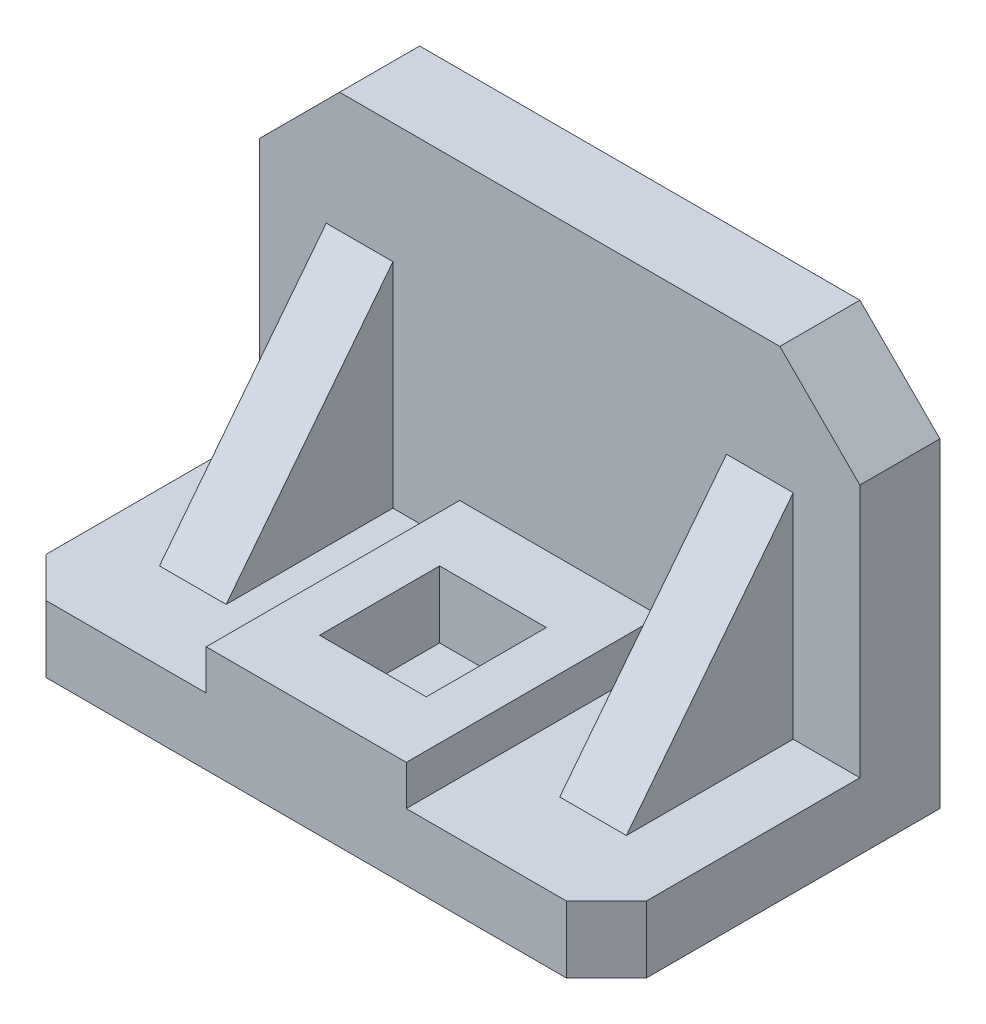
ISO-10303-21;
HEADER;
FILE_DESCRIPTION(('STEP AP214'),'2;1');
FILE_NAME('part.step','',(''),(''),'','','');
FILE_SCHEMA(('AUTOMOTIVE_DESIGN { 1 0 10303 214 1 1 1 1 }'));
ENDSEC;
DATA;
#1=APPLICATION_CONTEXT('core data for automotive mechanical design processes');
#2=APPLICATION_PROTOCOL_DEFINITION('international standard','automotive_design',2000,#1);
#3=PRODUCT_CONTEXT('',#1,'mechanical');
#4=PRODUCT('Part','Part','',(#3));
#5=PRODUCT_RELATED_PRODUCT_CATEGORY('part','',(#4));
#6=PRODUCT_DEFINITION_FORMATION('','',#4);
#7=PRODUCT_DEFINITION_CONTEXT('part definition',#1,'design');
#8=PRODUCT_DEFINITION('design','',#6,#7);
#9=PRODUCT_DEFINITION_SHAPE('','',#8);
#10=(LENGTH_UNIT() NAMED_UNIT(*) SI_UNIT(.MILLI.,.METRE.));
#11=(NAMED_UNIT(*) PLANE_ANGLE_UNIT() SI_UNIT($,.RADIAN.));
#12=(NAMED_UNIT(*) SI_UNIT($,.STERADIAN.) SOLID_ANGLE_UNIT());
#13=UNCERTAINTY_MEASURE_WITH_UNIT(LENGTH_MEASURE(1.E-05),#10,'distance_accuracy_value','');
#14=(GEOMETRIC_REPRESENTATION_CONTEXT(3) GLOBAL_UNCERTAINTY_ASSIGNED_CONTEXT((#13)) GLOBAL_UNIT_ASSIGNED_CONTEXT((#10,
#11,#12)) REPRESENTATION_CONTEXT('',''));
#15=CARTESIAN_POINT('',(0.,0.,0.));
#16=DIRECTION('',(0.,0.,1.));
#17=DIRECTION('',(1.,0.,0.));
#18=AXIS2_PLACEMENT_3D('',#15,#16,#17);
#19=CARTESIAN_POINT('',(70.,10.,37.));
#20=DIRECTION('',(0.,0.615644041972315,0.788024373724563));
#21=DIRECTION('',(0.,-0.788024373724563,0.615644041972315));
#22=AXIS2_PLACEMENT_3D('',#19,#20,#21);
#23=PLANE('',#22);
#24=DIRECTION('',(1.,0.,0.));
#25=VECTOR('',#24,1.);
#26=CARTESIAN_POINT('',(70.,10.,37.));
#27=LINE('',#26,#25);
#28=CARTESIAN_POINT('',(70.,10.,37.));
#29=VERTEX_POINT('',#28);
#30=CARTESIAN_POINT('',(80.,10.,37.));
#31=VERTEX_POINT('',#30);
#32=EDGE_CURVE('E422',#29,#31,#27,.T.);
#33=ORIENTED_EDGE('',*,*,#32,.T.);
#34=DIRECTION('',(0.,-0.788024373724563,0.615644041972315));
#35=VECTOR('',#34,1.);
#36=CARTESIAN_POINT('',(80.,10.,37.));
#37=LINE('',#36,#35);
#38=CARTESIAN_POINT('',(80.,42.,12.));
#39=VERTEX_POINT('',#38);
#40=EDGE_CURVE('E441',#39,#31,#37,.T.);
#41=ORIENTED_EDGE('',*,*,#40,.F.);
#42=DIRECTION('',(1.,0.,0.));
#43=VECTOR('',#42,1.);
#44=CARTESIAN_POINT('',(70.,42.,12.));
#45=LINE('',#44,#43);
#46=CARTESIAN_POINT('',(70.,42.,12.));
#47=VERTEX_POINT('',#46);
#48=EDGE_CURVE('E424',#47,#39,#45,.T.);
#49=ORIENTED_EDGE('',*,*,#48,.F.);
#50=DIRECTION('',(0.,-0.788024373724563,0.615644041972315));
#51=VECTOR('',#50,1.);
#52=CARTESIAN_POINT('',(70.,10.,37.));
#53=LINE('',#52,#51);
#54=EDGE_CURVE('E426',#47,#29,#53,.T.);
#55=ORIENTED_EDGE('',*,*,#54,.T.);
#56=EDGE_LOOP('',(#33,#41,#49,#55));
#57=FACE_BOUND('',#56,.T.);
#58=ADVANCED_FACE('F44',(#57),#23,.T.);
#59=CARTESIAN_POINT('',(0.,0.,12.));
#60=DIRECTION('',(0.,0.,-1.));
#61=DIRECTION('',(-1.,0.,0.));
#62=AXIS2_PLACEMENT_3D('',#59,#60,#61);
#63=PLANE('',#62);
#64=DIRECTION('',(0.,1.,0.));
#65=VECTOR('',#64,1.);
#66=CARTESIAN_POINT('',(70.,10.,12.));
#67=LINE('',#66,#65);
#68=CARTESIAN_POINT('',(70.,10.,12.));
#69=VERTEX_POINT('',#68);
#70=EDGE_CURVE('E433',#69,#47,#67,.T.);
#71=ORIENTED_EDGE('',*,*,#70,.T.);
#72=ORIENTED_EDGE('',*,*,#48,.T.);
#73=DIRECTION('',(0.,1.,0.));
#74=VECTOR('',#73,1.);
#75=CARTESIAN_POINT('',(80.,42.,12.));
#76=LINE('',#75,#74);
#77=CARTESIAN_POINT('',(80.,10.,12.));
#78=VERTEX_POINT('',#77);
#79=EDGE_CURVE('E70',#78,#39,#76,.T.);
#80=ORIENTED_EDGE('',*,*,#79,.F.);
#81=DIRECTION('',(1.,0.,0.));
#82=VECTOR('',#81,1.);
#83=CARTESIAN_POINT('',(80.,10.,12.));
#84=LINE('',#83,#82);
#85=CARTESIAN_POINT('',(90.,10.,12.));
#86=VERTEX_POINT('',#85);
#87=EDGE_CURVE('E381',#78,#86,#84,.T.);
#88=ORIENTED_EDGE('',*,*,#87,.T.);
#89=DIRECTION('',(0.,1.,0.));
#90=VECTOR('',#89,1.);
#91=CARTESIAN_POINT('',(90.,48.,12.));
#92=LINE('',#91,#90);
#93=CARTESIAN_POINT('',(90.,48.,12.));
#94=VERTEX_POINT('',#93);
#95=EDGE_CURVE('E326',#86,#94,#92,.T.);
#96=ORIENTED_EDGE('',*,*,#95,.T.);
#97=DIRECTION('',(-0.707106781186548,0.707106781186547,0.));
#98=VECTOR('',#97,1.);
#99=CARTESIAN_POINT('',(90.,48.,12.));
#100=LINE('',#99,#98);
#101=CARTESIAN_POINT('',(78.,60.,12.));
#102=VERTEX_POINT('',#101);
#103=EDGE_CURVE('E328',#94,#102,#100,.T.);
#104=ORIENTED_EDGE('',*,*,#103,.T.);
#105=DIRECTION('',(-1.,0.,0.));
#106=VECTOR('',#105,1.);
#107=CARTESIAN_POINT('',(12.,60.,12.));
#108=LINE('',#107,#106);
#109=CARTESIAN_POINT('',(12.,60.,12.));
#110=VERTEX_POINT('',#109);
#111=EDGE_CURVE('E335',#102,#110,#108,.T.);
#112=ORIENTED_EDGE('',*,*,#111,.T.);
#113=DIRECTION('',(-0.707106781186548,-0.707106781186548,0.));
#114=VECTOR('',#113,1.);
#115=CARTESIAN_POINT('',(0.,48.,12.));
#116=LINE('',#115,#114);
#117=CARTESIAN_POINT('',(0.,48.,12.));
#118=VERTEX_POINT('',#117);
#119=EDGE_CURVE('E332',#110,#118,#116,.T.);
#120=ORIENTED_EDGE('',*,*,#119,.T.);
#121=DIRECTION('',(0.,-1.,0.));
#122=VECTOR('',#121,1.);
#123=CARTESIAN_POINT('',(0.,0.,12.));
#124=LINE('',#123,#122);
#125=CARTESIAN_POINT('',(0.,10.,12.));
#126=VERTEX_POINT('',#125);
#127=EDGE_CURVE('E337',#118,#126,#124,.T.);
#128=ORIENTED_EDGE('',*,*,#127,.T.);
#129=DIRECTION('',(-1.,0.,0.));
#130=VECTOR('',#129,1.);
#131=CARTESIAN_POINT('',(10.,10.,12.));
#132=LINE('',#131,#130);
#133=CARTESIAN_POINT('',(10.,10.,12.));
#134=VERTEX_POINT('',#133);
#135=EDGE_CURVE('E213',#134,#126,#132,.T.);
#136=ORIENTED_EDGE('',*,*,#135,.F.);
#137=DIRECTION('',(0.,-1.,0.));
#138=VECTOR('',#137,1.);
#139=CARTESIAN_POINT('',(10.,42.,12.));
#140=LINE('',#139,#138);
#141=CARTESIAN_POINT('',(10.,42.,12.));
#142=VERTEX_POINT('',#141);
#143=EDGE_CURVE('E206',#142,#134,#140,.T.);
#144=ORIENTED_EDGE('',*,*,#143,.F.);
#145=DIRECTION('',(-1.,0.,0.));
#146=VECTOR('',#145,1.);
#147=CARTESIAN_POINT('',(20.,42.,12.));
#148=LINE('',#147,#146);
#149=CARTESIAN_POINT('',(20.,42.,12.));
#150=VERTEX_POINT('',#149);
#151=EDGE_CURVE('E212',#150,#142,#148,.T.);
#152=ORIENTED_EDGE('',*,*,#151,.F.);
#153=DIRECTION('',(0.,-1.,0.));
#154=VECTOR('',#153,1.);
#155=CARTESIAN_POINT('',(20.,10.,12.));
#156=LINE('',#155,#154);
#157=CARTESIAN_POINT('',(20.,10.,12.));
#158=VERTEX_POINT('',#157);
#159=EDGE_CURVE('E235',#150,#158,#156,.T.);
#160=ORIENTED_EDGE('',*,*,#159,.T.);
#161=DIRECTION('',(1.,0.,0.));
#162=VECTOR('',#161,1.);
#163=CARTESIAN_POINT('',(90.,10.,12.));
#164=LINE('',#163,#162);
#165=CARTESIAN_POINT('',(30.,10.,12.));
#166=VERTEX_POINT('',#165);
#167=EDGE_CURVE('E294',#158,#166,#164,.T.);
#168=ORIENTED_EDGE('',*,*,#167,.T.);
#169=DIRECTION('',(0.,-1.,0.));
#170=VECTOR('',#169,1.);
#171=CARTESIAN_POINT('',(30.,16.,12.));
#172=LINE('',#171,#170);
#173=CARTESIAN_POINT('',(30.,16.,12.));
#174=VERTEX_POINT('',#173);
#175=EDGE_CURVE('E280',#174,#166,#172,.T.);
#176=ORIENTED_EDGE('',*,*,#175,.F.);
#177=DIRECTION('',(-1.,0.,0.));
#178=VECTOR('',#177,1.);
#179=CARTESIAN_POINT('',(30.,16.,12.));
#180=LINE('',#179,#178);
#181=CARTESIAN_POINT('',(60.,16.,12.));
#182=VERTEX_POINT('',#181);
#183=EDGE_CURVE('E273',#182,#174,#180,.T.);
#184=ORIENTED_EDGE('',*,*,#183,.F.);
#185=DIRECTION('',(0.,-1.,0.));
#186=VECTOR('',#185,1.);
#187=CARTESIAN_POINT('',(60.,16.,12.));
#188=LINE('',#187,#186);
#189=CARTESIAN_POINT('',(60.,10.,12.));
#190=VERTEX_POINT('',#189);
#191=EDGE_CURVE('E285',#182,#190,#188,.T.);
#192=ORIENTED_EDGE('',*,*,#191,.T.);
#193=EDGE_CURVE('E291',#190,#69,#164,.T.);
#194=ORIENTED_EDGE('',*,*,#193,.T.);
#195=EDGE_LOOP('',(#71,#72,#80,#88,#96,#104,#112,#120,#128,#136,#144,#152,#160,#168,#176,#184,
#192,#194));
#196=FACE_BOUND('',#195,.T.);
#197=ADVANCED_FACE('F209',(#196),#63,.F.);
#198=CARTESIAN_POINT('',(0.,10.,0.));
#199=DIRECTION('',(0.,1.,0.));
#200=DIRECTION('',(0.,0.,1.));
#201=AXIS2_PLACEMENT_3D('',#198,#199,#200);
#202=PLANE('',#201);
#203=DIRECTION('',(-1.,0.,0.));
#204=VECTOR('',#203,1.);
#205=CARTESIAN_POINT('',(20.,10.,37.));
#206=LINE('',#205,#204);
#207=CARTESIAN_POINT('',(20.,10.,37.));
#208=VERTEX_POINT('',#207);
#209=CARTESIAN_POINT('',(10.,10.,37.));
#210=VERTEX_POINT('',#209);
#211=EDGE_CURVE('E226',#208,#210,#206,.T.);
#212=ORIENTED_EDGE('',*,*,#211,.T.);
#213=DIRECTION('',(0.,0.,1.));
#214=VECTOR('',#213,1.);
#215=CARTESIAN_POINT('',(10.,10.,12.));
#216=LINE('',#215,#214);
#217=EDGE_CURVE('E58',#134,#210,#216,.T.);
#218=ORIENTED_EDGE('',*,*,#217,.F.);
#219=ORIENTED_EDGE('',*,*,#135,.T.);
#220=DIRECTION('',(0.,0.,-1.));
#221=VECTOR('',#220,1.);
#222=CARTESIAN_POINT('',(0.,10.,12.));
#223=LINE('',#222,#221);
#224=CARTESIAN_POINT('',(0.,10.,44.));
#225=VERTEX_POINT('',#224);
#226=EDGE_CURVE('E293',#225,#126,#223,.T.);
#227=ORIENTED_EDGE('',*,*,#226,.F.);
#228=DIRECTION('',(-0.707106781186547,0.,-0.707106781186548));
#229=VECTOR('',#228,1.);
#230=CARTESIAN_POINT('',(0.,10.,44.));
#231=LINE('',#230,#229);
#232=CARTESIAN_POINT('',(6.,10.,50.));
#233=VERTEX_POINT('',#232);
#234=EDGE_CURVE('E306',#233,#225,#231,.T.);
#235=ORIENTED_EDGE('',*,*,#234,.F.);
#236=DIRECTION('',(-1.,0.,0.));
#237=VECTOR('',#236,1.);
#238=CARTESIAN_POINT('',(6.,10.,50.));
#239=LINE('',#238,#237);
#240=CARTESIAN_POINT('',(30.,10.,50.));
#241=VERTEX_POINT('',#240);
#242=EDGE_CURVE('E305',#241,#233,#239,.T.);
#243=ORIENTED_EDGE('',*,*,#242,.F.);
#244=DIRECTION('',(0.,0.,1.));
#245=VECTOR('',#244,1.);
#246=CARTESIAN_POINT('',(30.,10.,12.));
#247=LINE('',#246,#245);
#248=EDGE_CURVE('E258',#166,#241,#247,.T.);
#249=ORIENTED_EDGE('',*,*,#248,.F.);
#250=ORIENTED_EDGE('',*,*,#167,.F.);
#251=DIRECTION('',(0.,0.,1.));
#252=VECTOR('',#251,1.);
#253=CARTESIAN_POINT('',(20.,10.,12.));
#254=LINE('',#253,#252);
#255=EDGE_CURVE('E423',#158,#208,#254,.T.);
#256=ORIENTED_EDGE('',*,*,#255,.T.);
#257=EDGE_LOOP('',(#212,#218,#219,#227,#235,#243,#249,#250,#256));
#258=FACE_BOUND('',#257,.T.);
#259=ADVANCED_FACE('F401',(#258),#202,.T.);
#260=ORIENTED_EDGE('',*,*,#32,.F.);
#261=DIRECTION('',(0.,0.,-1.));
#262=VECTOR('',#261,1.);
#263=CARTESIAN_POINT('',(70.,10.,12.));
#264=LINE('',#263,#262);
#265=EDGE_CURVE('E434',#29,#69,#264,.T.);
#266=ORIENTED_EDGE('',*,*,#265,.T.);
#267=ORIENTED_EDGE('',*,*,#193,.F.);
#268=DIRECTION('',(0.,0.,-1.));
#269=VECTOR('',#268,1.);
#270=CARTESIAN_POINT('',(60.,10.,12.));
#271=LINE('',#270,#269);
#272=CARTESIAN_POINT('',(60.,10.,50.));
#273=VERTEX_POINT('',#272);
#274=EDGE_CURVE('E272',#273,#190,#271,.T.);
#275=ORIENTED_EDGE('',*,*,#274,.F.);
#276=CARTESIAN_POINT('',(84.,10.,50.));
#277=VERTEX_POINT('',#276);
#278=EDGE_CURVE('E303',#277,#273,#239,.T.);
#279=ORIENTED_EDGE('',*,*,#278,.F.);
#280=DIRECTION('',(-0.707106781186547,0.,0.707106781186547));
#281=VECTOR('',#280,1.);
#282=CARTESIAN_POINT('',(90.,10.,44.));
#283=LINE('',#282,#281);
#284=CARTESIAN_POINT('',(90.,10.,44.));
#285=VERTEX_POINT('',#284);
#286=EDGE_CURVE('E299',#285,#277,#283,.T.);
#287=ORIENTED_EDGE('',*,*,#286,.F.);
#288=DIRECTION('',(0.,0.,1.));
#289=VECTOR('',#288,1.);
#290=CARTESIAN_POINT('',(90.,10.,12.));
#291=LINE('',#290,#289);
#292=EDGE_CURVE('E300',#86,#285,#291,.T.);
#293=ORIENTED_EDGE('',*,*,#292,.F.);
#294=ORIENTED_EDGE('',*,*,#87,.F.);
#295=DIRECTION('',(0.,0.,-1.));
#296=VECTOR('',#295,1.);
#297=CARTESIAN_POINT('',(80.,10.,12.));
#298=LINE('',#297,#296);
#299=EDGE_CURVE('E437',#31,#78,#298,.T.);
#300=ORIENTED_EDGE('',*,*,#299,.F.);
#301=EDGE_LOOP('',(#260,#266,#267,#275,#279,#287,#293,#294,#300));
#302=FACE_BOUND('',#301,.T.);
#303=ADVANCED_FACE('F388',(#302),#202,.T.);
#304=CARTESIAN_POINT('',(90.,0.,12.));
#305=DIRECTION('',(0.,1.,0.));
#306=DIRECTION('',(0.,0.,1.));
#307=AXIS2_PLACEMENT_3D('',#304,#305,#306);
#308=PLANE('',#307);
#309=DIRECTION('',(1.,0.,0.));
#310=VECTOR('',#309,1.);
#311=CARTESIAN_POINT('',(90.,0.,0.));
#312=LINE('',#311,#310);
#313=CARTESIAN_POINT('',(0.,0.,0.));
#314=VERTEX_POINT('',#313);
#315=CARTESIAN_POINT('',(90.,0.,0.));
#316=VERTEX_POINT('',#315);
#317=EDGE_CURVE('E318',#314,#316,#312,.T.);
#318=ORIENTED_EDGE('',*,*,#317,.T.);
#319=DIRECTION('',(0.,0.,-1.));
#320=VECTOR('',#319,1.);
#321=CARTESIAN_POINT('',(90.,0.,12.));
#322=LINE('',#321,#320);
#323=CARTESIAN_POINT('',(90.,0.,44.));
#324=VERTEX_POINT('',#323);
#325=EDGE_CURVE('E11',#324,#316,#322,.T.);
#326=ORIENTED_EDGE('',*,*,#325,.F.);
#327=DIRECTION('',(-0.707106781186547,0.,0.707106781186547));
#328=VECTOR('',#327,1.);
#329=CARTESIAN_POINT('',(90.,0.,44.));
#330=LINE('',#329,#328);
#331=CARTESIAN_POINT('',(84.,0.,50.));
#332=VERTEX_POINT('',#331);
#333=EDGE_CURVE('E289',#324,#332,#330,.T.);
#334=ORIENTED_EDGE('',*,*,#333,.T.);
#335=DIRECTION('',(-1.,0.,0.));
#336=VECTOR('',#335,1.);
#337=CARTESIAN_POINT('',(6.,0.,50.));
#338=LINE('',#337,#336);
#339=CARTESIAN_POINT('',(6.,0.,50.));
#340=VERTEX_POINT('',#339);
#341=EDGE_CURVE('E315',#332,#340,#338,.T.);
#342=ORIENTED_EDGE('',*,*,#341,.T.);
#343=DIRECTION('',(-0.707106781186547,0.,-0.707106781186548));
#344=VECTOR('',#343,1.);
#345=CARTESIAN_POINT('',(0.,0.,44.));
#346=LINE('',#345,#344);
#347=CARTESIAN_POINT('',(0.,0.,44.));
#348=VERTEX_POINT('',#347);
#349=EDGE_CURVE('E295',#340,#348,#346,.T.);
#350=ORIENTED_EDGE('',*,*,#349,.T.);
#351=DIRECTION('',(0.,0.,-1.));
#352=VECTOR('',#351,1.);
#353=CARTESIAN_POINT('',(0.,0.,12.));
#354=LINE('',#353,#352);
#355=EDGE_CURVE('E336',#348,#314,#354,.T.);
#356=ORIENTED_EDGE('',*,*,#355,.T.);
#357=EDGE_LOOP('',(#318,#326,#334,#342,#350,#356));
#358=FACE_BOUND('',#357,.T.);
#359=ADVANCED_FACE('F50',(#358),#308,.F.);
#360=CARTESIAN_POINT('',(90.,48.,12.));
#361=DIRECTION('',(-1.,0.,0.));
#362=DIRECTION('',(0.,0.,1.));
#363=AXIS2_PLACEMENT_3D('',#360,#361,#362);
#364=PLANE('',#363);
#365=ORIENTED_EDGE('',*,*,#95,.F.);
#366=ORIENTED_EDGE('',*,*,#292,.T.);
#367=DIRECTION('',(0.,-1.,0.));
#368=VECTOR('',#367,1.);
#369=CARTESIAN_POINT('',(90.,10.,44.));
#370=LINE('',#369,#368);
#371=EDGE_CURVE('E307',#285,#324,#370,.T.);
#372=ORIENTED_EDGE('',*,*,#371,.T.);
#373=ORIENTED_EDGE('',*,*,#325,.T.);
#374=DIRECTION('',(0.,1.,0.));
#375=VECTOR('',#374,1.);
#376=CARTESIAN_POINT('',(90.,48.,0.));
#377=LINE('',#376,#375);
#378=CARTESIAN_POINT('',(90.,48.,0.));
#379=VERTEX_POINT('',#378);
#380=EDGE_CURVE('E342',#316,#379,#377,.T.);
#381=ORIENTED_EDGE('',*,*,#380,.T.);
#382=DIRECTION('',(0.,0.,-1.));
#383=VECTOR('',#382,1.);
#384=CARTESIAN_POINT('',(90.,48.,12.));
#385=LINE('',#384,#383);
#386=EDGE_CURVE('E52',#94,#379,#385,.T.);
#387=ORIENTED_EDGE('',*,*,#386,.F.);
#388=EDGE_LOOP('',(#365,#366,#372,#373,#381,#387));
#389=FACE_BOUND('',#388,.T.);
#390=ADVANCED_FACE('F387',(#389),#364,.F.);
#391=CARTESIAN_POINT('',(90.,48.,12.));
#392=DIRECTION('',(-0.707106781186547,-0.707106781186548,0.));
#393=DIRECTION('',(0.707106781186548,-0.707106781186547,0.));
#394=AXIS2_PLACEMENT_3D('',#391,#392,#393);
#395=PLANE('',#394);
#396=DIRECTION('',(-0.707106781186548,0.707106781186547,0.));
#397=VECTOR('',#396,1.);
#398=CARTESIAN_POINT('',(90.,48.,0.));
#399=LINE('',#398,#397);
#400=CARTESIAN_POINT('',(78.,60.,0.));
#401=VERTEX_POINT('',#400);
#402=EDGE_CURVE('E344',#379,#401,#399,.T.);
#403=ORIENTED_EDGE('',*,*,#402,.T.);
#404=DIRECTION('',(0.,0.,-1.));
#405=VECTOR('',#404,1.);
#406=CARTESIAN_POINT('',(78.,60.,12.));
#407=LINE('',#406,#405);
#408=EDGE_CURVE('E356',#102,#401,#407,.T.);
#409=ORIENTED_EDGE('',*,*,#408,.F.);
#410=ORIENTED_EDGE('',*,*,#103,.F.);
#411=ORIENTED_EDGE('',*,*,#386,.T.);
#412=EDGE_LOOP('',(#403,#409,#410,#411));
#413=FACE_BOUND('',#412,.T.);
#414=ADVANCED_FACE('F362',(#413),#395,.F.);
#415=CARTESIAN_POINT('',(12.,60.,12.));
#416=DIRECTION('',(0.,-1.,0.));
#417=DIRECTION('',(0.,0.,-1.));
#418=AXIS2_PLACEMENT_3D('',#415,#416,#417);
#419=PLANE('',#418);
#420=DIRECTION('',(-1.,0.,0.));
#421=VECTOR('',#420,1.);
#422=CARTESIAN_POINT('',(12.,60.,0.));
#423=LINE('',#422,#421);
#424=CARTESIAN_POINT('',(12.,60.,0.));
#425=VERTEX_POINT('',#424);
#426=EDGE_CURVE('E343',#401,#425,#423,.T.);
#427=ORIENTED_EDGE('',*,*,#426,.T.);
#428=DIRECTION('',(0.,0.,-1.));
#429=VECTOR('',#428,1.);
#430=CARTESIAN_POINT('',(12.,60.,12.));
#431=LINE('',#430,#429);
#432=EDGE_CURVE('E354',#110,#425,#431,.T.);
#433=ORIENTED_EDGE('',*,*,#432,.F.);
#434=ORIENTED_EDGE('',*,*,#111,.F.);
#435=ORIENTED_EDGE('',*,*,#408,.T.);
#436=EDGE_LOOP('',(#427,#433,#434,#435));
#437=FACE_BOUND('',#436,.T.);
#438=ADVANCED_FACE('F376',(#437),#419,.F.);
#439=CARTESIAN_POINT('',(0.,48.,12.));
#440=DIRECTION('',(0.707106781186547,-0.707106781186547,0.));
#441=DIRECTION('',(0.707106781186548,0.707106781186548,0.));
#442=AXIS2_PLACEMENT_3D('',#439,#440,#441);
#443=PLANE('',#442);
#444=DIRECTION('',(-0.707106781186548,-0.707106781186548,0.));
#445=VECTOR('',#444,1.);
#446=CARTESIAN_POINT('',(0.,48.,0.));
#447=LINE('',#446,#445);
#448=CARTESIAN_POINT('',(0.,48.,0.));
#449=VERTEX_POINT('',#448);
#450=EDGE_CURVE('E346',#425,#449,#447,.T.);
#451=ORIENTED_EDGE('',*,*,#450,.T.);
#452=DIRECTION('',(0.,0.,-1.));
#453=VECTOR('',#452,1.);
#454=CARTESIAN_POINT('',(0.,48.,12.));
#455=LINE('',#454,#453);
#456=EDGE_CURVE('E355',#118,#449,#455,.T.);
#457=ORIENTED_EDGE('',*,*,#456,.F.);
#458=ORIENTED_EDGE('',*,*,#119,.F.);
#459=ORIENTED_EDGE('',*,*,#432,.T.);
#460=EDGE_LOOP('',(#451,#457,#458,#459));
#461=FACE_BOUND('',#460,.T.);
#462=ADVANCED_FACE('F379',(#461),#443,.F.);
#463=CARTESIAN_POINT('',(0.,0.,12.));
#464=DIRECTION('',(1.,0.,0.));
#465=DIRECTION('',(0.,0.,-1.));
#466=AXIS2_PLACEMENT_3D('',#463,#464,#465);
#467=PLANE('',#466);
#468=ORIENTED_EDGE('',*,*,#226,.T.);
#469=ORIENTED_EDGE('',*,*,#127,.F.);
#470=ORIENTED_EDGE('',*,*,#456,.T.);
#471=DIRECTION('',(0.,-1.,0.));
#472=VECTOR('',#471,1.);
#473=CARTESIAN_POINT('',(0.,0.,0.));
#474=LINE('',#473,#472);
#475=EDGE_CURVE('E327',#449,#314,#474,.T.);
#476=ORIENTED_EDGE('',*,*,#475,.T.);
#477=ORIENTED_EDGE('',*,*,#355,.F.);
#478=DIRECTION('',(0.,-1.,0.));
#479=VECTOR('',#478,1.);
#480=CARTESIAN_POINT('',(0.,10.,44.));
#481=LINE('',#480,#479);
#482=EDGE_CURVE('E320',#225,#348,#481,.T.);
#483=ORIENTED_EDGE('',*,*,#482,.F.);
#484=EDGE_LOOP('',(#468,#469,#470,#476,#477,#483));
#485=FACE_BOUND('',#484,.T.);
#486=ADVANCED_FACE('F397',(#485),#467,.F.);
#487=CARTESIAN_POINT('',(0.,0.,0.));
#488=DIRECTION('',(0.,0.,-1.));
#489=DIRECTION('',(-1.,0.,0.));
#490=AXIS2_PLACEMENT_3D('',#487,#488,#489);
#491=PLANE('',#490);
#492=ORIENTED_EDGE('',*,*,#317,.F.);
#493=ORIENTED_EDGE('',*,*,#475,.F.);
#494=ORIENTED_EDGE('',*,*,#450,.F.);
#495=ORIENTED_EDGE('',*,*,#426,.F.);
#496=ORIENTED_EDGE('',*,*,#402,.F.);
#497=ORIENTED_EDGE('',*,*,#380,.F.);
#498=EDGE_LOOP('',(#492,#493,#494,#495,#496,#497));
#499=FACE_BOUND('',#498,.T.);
#500=ADVANCED_FACE('F371',(#499),#491,.T.);
#501=CARTESIAN_POINT('',(0.,10.,44.));
#502=DIRECTION('',(-0.707106781186548,0.,0.707106781186547));
#503=DIRECTION('',(0.707106781186547,0.,0.707106781186548));
#504=AXIS2_PLACEMENT_3D('',#501,#502,#503);
#505=PLANE('',#504);
#506=ORIENTED_EDGE('',*,*,#349,.F.);
#507=DIRECTION('',(0.,-1.,0.));
#508=VECTOR('',#507,1.);
#509=CARTESIAN_POINT('',(6.,10.,50.));
#510=LINE('',#509,#508);
#511=EDGE_CURVE('E322',#233,#340,#510,.T.);
#512=ORIENTED_EDGE('',*,*,#511,.F.);
#513=ORIENTED_EDGE('',*,*,#234,.T.);
#514=ORIENTED_EDGE('',*,*,#482,.T.);
#515=EDGE_LOOP('',(#506,#512,#513,#514));
#516=FACE_BOUND('',#515,.T.);
#517=ADVANCED_FACE('F409',(#516),#505,.T.);
#518=CARTESIAN_POINT('',(6.,10.,50.));
#519=DIRECTION('',(0.,0.,1.));
#520=DIRECTION('',(1.,0.,0.));
#521=AXIS2_PLACEMENT_3D('',#518,#519,#520);
#522=PLANE('',#521);
#523=ORIENTED_EDGE('',*,*,#341,.F.);
#524=DIRECTION('',(0.,-1.,0.));
#525=VECTOR('',#524,1.);
#526=CARTESIAN_POINT('',(84.,10.,50.));
#527=LINE('',#526,#525);
#528=EDGE_CURVE('E324',#277,#332,#527,.T.);
#529=ORIENTED_EDGE('',*,*,#528,.F.);
#530=ORIENTED_EDGE('',*,*,#278,.T.);
#531=DIRECTION('',(0.,-1.,0.));
#532=VECTOR('',#531,1.);
#533=CARTESIAN_POINT('',(60.,16.,50.));
#534=LINE('',#533,#532);
#535=CARTESIAN_POINT('',(60.,16.,50.));
#536=VERTEX_POINT('',#535);
#537=EDGE_CURVE('E286',#536,#273,#534,.T.);
#538=ORIENTED_EDGE('',*,*,#537,.F.);
#539=DIRECTION('',(1.,0.,0.));
#540=VECTOR('',#539,1.);
#541=CARTESIAN_POINT('',(30.,16.,50.));
#542=LINE('',#541,#540);
#543=CARTESIAN_POINT('',(30.,16.,50.));
#544=VERTEX_POINT('',#543);
#545=EDGE_CURVE('E269',#544,#536,#542,.T.);
#546=ORIENTED_EDGE('',*,*,#545,.F.);
#547=DIRECTION('',(0.,-1.,0.));
#548=VECTOR('',#547,1.);
#549=CARTESIAN_POINT('',(30.,16.,50.));
#550=LINE('',#549,#548);
#551=EDGE_CURVE('E288',#544,#241,#550,.T.);
#552=ORIENTED_EDGE('',*,*,#551,.T.);
#553=ORIENTED_EDGE('',*,*,#242,.T.);
#554=ORIENTED_EDGE('',*,*,#511,.T.);
#555=EDGE_LOOP('',(#523,#529,#530,#538,#546,#552,#553,#554));
#556=FACE_BOUND('',#555,.T.);
#557=ADVANCED_FACE('F408',(#556),#522,.T.);
#558=CARTESIAN_POINT('',(90.,10.,44.));
#559=DIRECTION('',(0.707106781186548,0.,0.707106781186548));
#560=DIRECTION('',(0.707106781186548,0.,-0.707106781186548));
#561=AXIS2_PLACEMENT_3D('',#558,#559,#560);
#562=PLANE('',#561);
#563=ORIENTED_EDGE('',*,*,#333,.F.);
#564=ORIENTED_EDGE('',*,*,#371,.F.);
#565=ORIENTED_EDGE('',*,*,#286,.T.);
#566=ORIENTED_EDGE('',*,*,#528,.T.);
#567=EDGE_LOOP('',(#563,#564,#565,#566));
#568=FACE_BOUND('',#567,.T.);
#569=ADVANCED_FACE('F392',(#568),#562,.T.);
#570=CARTESIAN_POINT('',(30.,16.,12.));
#571=DIRECTION('',(1.,0.,0.));
#572=DIRECTION('',(0.,0.,-1.));
#573=AXIS2_PLACEMENT_3D('',#570,#571,#572);
#574=PLANE('',#573);
#575=ORIENTED_EDGE('',*,*,#248,.T.);
#576=ORIENTED_EDGE('',*,*,#551,.F.);
#577=DIRECTION('',(0.,0.,1.));
#578=VECTOR('',#577,1.);
#579=CARTESIAN_POINT('',(30.,16.,12.));
#580=LINE('',#579,#578);
#581=EDGE_CURVE('E270',#174,#544,#580,.T.);
#582=ORIENTED_EDGE('',*,*,#581,.F.);
#583=ORIENTED_EDGE('',*,*,#175,.T.);
#584=EDGE_LOOP('',(#575,#576,#582,#583));
#585=FACE_BOUND('',#584,.T.);
#586=ADVANCED_FACE('F416',(#585),#574,.F.);
#587=CARTESIAN_POINT('',(60.,16.,12.));
#588=DIRECTION('',(-1.,0.,0.));
#589=DIRECTION('',(0.,0.,1.));
#590=AXIS2_PLACEMENT_3D('',#587,#588,#589);
#591=PLANE('',#590);
#592=ORIENTED_EDGE('',*,*,#274,.T.);
#593=ORIENTED_EDGE('',*,*,#191,.F.);
#594=DIRECTION('',(0.,0.,-1.));
#595=VECTOR('',#594,1.);
#596=CARTESIAN_POINT('',(60.,16.,12.));
#597=LINE('',#596,#595);
#598=EDGE_CURVE('E271',#536,#182,#597,.T.);
#599=ORIENTED_EDGE('',*,*,#598,.F.);
#600=ORIENTED_EDGE('',*,*,#537,.T.);
#601=EDGE_LOOP('',(#592,#593,#599,#600));
#602=FACE_BOUND('',#601,.T.);
#603=ADVANCED_FACE('F460',(#602),#591,.F.);
#604=CARTESIAN_POINT('',(0.,16.,0.));
#605=DIRECTION('',(0.,1.,0.));
#606=DIRECTION('',(0.,0.,1.));
#607=AXIS2_PLACEMENT_3D('',#604,#605,#606);
#608=PLANE('',#607);
#609=DIRECTION('',(0.,0.,1.));
#610=VECTOR('',#609,1.);
#611=CARTESIAN_POINT('',(37.,16.,22.));
#612=LINE('',#611,#610);
#613=CARTESIAN_POINT('',(37.,16.,22.));
#614=VERTEX_POINT('',#613);
#615=CARTESIAN_POINT('',(37.,16.,40.));
#616=VERTEX_POINT('',#615);
#617=EDGE_CURVE('E227',#614,#616,#612,.T.);
#618=ORIENTED_EDGE('',*,*,#617,.F.);
#619=DIRECTION('',(-1.,0.,0.));
#620=VECTOR('',#619,1.);
#621=CARTESIAN_POINT('',(37.,16.,22.));
#622=LINE('',#621,#620);
#623=CARTESIAN_POINT('',(53.,16.,22.));
#624=VERTEX_POINT('',#623);
#625=EDGE_CURVE('E241',#624,#614,#622,.T.);
#626=ORIENTED_EDGE('',*,*,#625,.F.);
#627=DIRECTION('',(0.,0.,-1.));
#628=VECTOR('',#627,1.);
#629=CARTESIAN_POINT('',(53.,16.,22.));
#630=LINE('',#629,#628);
#631=CARTESIAN_POINT('',(53.,16.,40.));
#632=VERTEX_POINT('',#631);
#633=EDGE_CURVE('E254',#632,#624,#630,.T.);
#634=ORIENTED_EDGE('',*,*,#633,.F.);
#635=DIRECTION('',(1.,0.,0.));
#636=VECTOR('',#635,1.);
#637=CARTESIAN_POINT('',(37.,16.,40.));
#638=LINE('',#637,#636);
#639=EDGE_CURVE('E229',#616,#632,#638,.T.);
#640=ORIENTED_EDGE('',*,*,#639,.F.);
#641=EDGE_LOOP('',(#618,#626,#634,#640));
#642=FACE_BOUND('',#641,.T.);
#643=ORIENTED_EDGE('',*,*,#581,.T.);
#644=ORIENTED_EDGE('',*,*,#545,.T.);
#645=ORIENTED_EDGE('',*,*,#598,.T.);
#646=ORIENTED_EDGE('',*,*,#183,.T.);
#647=EDGE_LOOP('',(#643,#644,#645,#646));
#648=FACE_BOUND('',#647,.T.);
#649=ADVANCED_FACE('F457',(#642,#648),#608,.T.);
#650=CARTESIAN_POINT('',(37.,6.,22.));
#651=DIRECTION('',(-1.,0.,0.));
#652=DIRECTION('',(0.,0.,1.));
#653=AXIS2_PLACEMENT_3D('',#650,#651,#652);
#654=PLANE('',#653);
#655=ORIENTED_EDGE('',*,*,#617,.T.);
#656=DIRECTION('',(0.,1.,0.));
#657=VECTOR('',#656,1.);
#658=CARTESIAN_POINT('',(37.,6.,40.));
#659=LINE('',#658,#657);
#660=CARTESIAN_POINT('',(37.,6.,40.));
#661=VERTEX_POINT('',#660);
#662=EDGE_CURVE('E248',#661,#616,#659,.T.);
#663=ORIENTED_EDGE('',*,*,#662,.F.);
#664=DIRECTION('',(0.,0.,1.));
#665=VECTOR('',#664,1.);
#666=CARTESIAN_POINT('',(37.,6.,22.));
#667=LINE('',#666,#665);
#668=CARTESIAN_POINT('',(37.,6.,22.));
#669=VERTEX_POINT('',#668);
#670=EDGE_CURVE('E240',#669,#661,#667,.T.);
#671=ORIENTED_EDGE('',*,*,#670,.F.);
#672=DIRECTION('',(0.,1.,0.));
#673=VECTOR('',#672,1.);
#674=CARTESIAN_POINT('',(37.,6.,22.));
#675=LINE('',#674,#673);
#676=EDGE_CURVE('E259',#669,#614,#675,.T.);
#677=ORIENTED_EDGE('',*,*,#676,.T.);
#678=EDGE_LOOP('',(#655,#663,#671,#677));
#679=FACE_BOUND('',#678,.T.);
#680=ADVANCED_FACE('F465',(#679),#654,.F.);
#681=CARTESIAN_POINT('',(37.,6.,22.));
#682=DIRECTION('',(0.,0.,-1.));
#683=DIRECTION('',(-1.,0.,0.));
#684=AXIS2_PLACEMENT_3D('',#681,#682,#683);
#685=PLANE('',#684);
#686=ORIENTED_EDGE('',*,*,#625,.T.);
#687=ORIENTED_EDGE('',*,*,#676,.F.);
#688=DIRECTION('',(-1.,0.,0.));
#689=VECTOR('',#688,1.);
#690=CARTESIAN_POINT('',(37.,6.,22.));
#691=LINE('',#690,#689);
#692=CARTESIAN_POINT('',(53.,6.,22.));
#693=VERTEX_POINT('',#692);
#694=EDGE_CURVE('E250',#693,#669,#691,.T.);
#695=ORIENTED_EDGE('',*,*,#694,.F.);
#696=DIRECTION('',(0.,1.,0.));
#697=VECTOR('',#696,1.);
#698=CARTESIAN_POINT('',(53.,6.,22.));
#699=LINE('',#698,#697);
#700=EDGE_CURVE('E264',#693,#624,#699,.T.);
#701=ORIENTED_EDGE('',*,*,#700,.T.);
#702=EDGE_LOOP('',(#686,#687,#695,#701));
#703=FACE_BOUND('',#702,.T.);
#704=ADVANCED_FACE('F468',(#703),#685,.F.);
#705=CARTESIAN_POINT('',(53.,6.,22.));
#706=DIRECTION('',(1.,0.,0.));
#707=DIRECTION('',(0.,0.,-1.));
#708=AXIS2_PLACEMENT_3D('',#705,#706,#707);
#709=PLANE('',#708);
#710=ORIENTED_EDGE('',*,*,#633,.T.);
#711=ORIENTED_EDGE('',*,*,#700,.F.);
#712=DIRECTION('',(0.,0.,-1.));
#713=VECTOR('',#712,1.);
#714=CARTESIAN_POINT('',(53.,6.,22.));
#715=LINE('',#714,#713);
#716=CARTESIAN_POINT('',(53.,6.,40.));
#717=VERTEX_POINT('',#716);
#718=EDGE_CURVE('E242',#717,#693,#715,.T.);
#719=ORIENTED_EDGE('',*,*,#718,.F.);
#720=DIRECTION('',(0.,1.,0.));
#721=VECTOR('',#720,1.);
#722=CARTESIAN_POINT('',(53.,6.,40.));
#723=LINE('',#722,#721);
#724=EDGE_CURVE('E265',#717,#632,#723,.T.);
#725=ORIENTED_EDGE('',*,*,#724,.T.);
#726=EDGE_LOOP('',(#710,#711,#719,#725));
#727=FACE_BOUND('',#726,.T.);
#728=ADVANCED_FACE('F496',(#727),#709,.F.);
#729=CARTESIAN_POINT('',(37.,6.,40.));
#730=DIRECTION('',(0.,0.,1.));
#731=DIRECTION('',(1.,0.,0.));
#732=AXIS2_PLACEMENT_3D('',#729,#730,#731);
#733=PLANE('',#732);
#734=ORIENTED_EDGE('',*,*,#639,.T.);
#735=ORIENTED_EDGE('',*,*,#724,.F.);
#736=DIRECTION('',(1.,0.,0.));
#737=VECTOR('',#736,1.);
#738=CARTESIAN_POINT('',(37.,6.,40.));
#739=LINE('',#738,#737);
#740=EDGE_CURVE('E239',#661,#717,#739,.T.);
#741=ORIENTED_EDGE('',*,*,#740,.F.);
#742=ORIENTED_EDGE('',*,*,#662,.T.);
#743=EDGE_LOOP('',(#734,#735,#741,#742));
#744=FACE_BOUND('',#743,.T.);
#745=ADVANCED_FACE('F495',(#744),#733,.F.);
#746=CARTESIAN_POINT('',(0.,6.,0.));
#747=DIRECTION('',(0.,1.,0.));
#748=DIRECTION('',(0.,0.,1.));
#749=AXIS2_PLACEMENT_3D('',#746,#747,#748);
#750=PLANE('',#749);
#751=ORIENTED_EDGE('',*,*,#670,.T.);
#752=ORIENTED_EDGE('',*,*,#740,.T.);
#753=ORIENTED_EDGE('',*,*,#718,.T.);
#754=ORIENTED_EDGE('',*,*,#694,.T.);
#755=EDGE_LOOP('',(#751,#752,#753,#754));
#756=FACE_BOUND('',#755,.T.);
#757=ADVANCED_FACE('F490',(#756),#750,.T.);
#758=CARTESIAN_POINT('',(20.,10.,37.));
#759=DIRECTION('',(0.,0.615644041972315,0.788024373724563));
#760=DIRECTION('',(0.,-0.788024373724563,0.615644041972315));
#761=AXIS2_PLACEMENT_3D('',#758,#759,#760);
#762=PLANE('',#761);
#763=DIRECTION('',(0.,0.788024373724563,-0.615644041972315));
#764=VECTOR('',#763,1.);
#765=CARTESIAN_POINT('',(10.,10.,37.));
#766=LINE('',#765,#764);
#767=EDGE_CURVE('E219',#210,#142,#766,.T.);
#768=ORIENTED_EDGE('',*,*,#767,.F.);
#769=ORIENTED_EDGE('',*,*,#211,.F.);
#770=DIRECTION('',(0.,0.788024373724563,-0.615644041972315));
#771=VECTOR('',#770,1.);
#772=CARTESIAN_POINT('',(20.,10.,37.));
#773=LINE('',#772,#771);
#774=EDGE_CURVE('E224',#208,#150,#773,.T.);
#775=ORIENTED_EDGE('',*,*,#774,.T.);
#776=ORIENTED_EDGE('',*,*,#151,.T.);
#777=EDGE_LOOP('',(#768,#769,#775,#776));
#778=FACE_BOUND('',#777,.T.);
#779=ADVANCED_FACE('F223',(#778),#762,.T.);
#780=CARTESIAN_POINT('',(20.,0.,0.));
#781=DIRECTION('',(-1.,0.,0.));
#782=DIRECTION('',(0.,0.,1.));
#783=AXIS2_PLACEMENT_3D('',#780,#781,#782);
#784=PLANE('',#783);
#785=ORIENTED_EDGE('',*,*,#255,.F.);
#786=ORIENTED_EDGE('',*,*,#159,.F.);
#787=ORIENTED_EDGE('',*,*,#774,.F.);
#788=EDGE_LOOP('',(#785,#786,#787));
#789=FACE_BOUND('',#788,.T.);
#790=ADVANCED_FACE('F482',(#789),#784,.F.);
#791=CARTESIAN_POINT('',(70.,0.,0.));
#792=DIRECTION('',(-1.,0.,0.));
#793=DIRECTION('',(0.,0.,1.));
#794=AXIS2_PLACEMENT_3D('',#791,#792,#793);
#795=PLANE('',#794);
#796=ORIENTED_EDGE('',*,*,#265,.F.);
#797=ORIENTED_EDGE('',*,*,#54,.F.);
#798=ORIENTED_EDGE('',*,*,#70,.F.);
#799=EDGE_LOOP('',(#796,#797,#798));
#800=FACE_BOUND('',#799,.T.);
#801=ADVANCED_FACE('F454',(#800),#795,.T.);
#802=CARTESIAN_POINT('',(80.,0.,0.));
#803=DIRECTION('',(1.,0.,0.));
#804=DIRECTION('',(0.,0.,-1.));
#805=AXIS2_PLACEMENT_3D('',#802,#803,#804);
#806=PLANE('',#805);
#807=ORIENTED_EDGE('',*,*,#40,.T.);
#808=ORIENTED_EDGE('',*,*,#299,.T.);
#809=ORIENTED_EDGE('',*,*,#79,.T.);
#810=EDGE_LOOP('',(#807,#808,#809));
#811=FACE_BOUND('',#810,.T.);
#812=ADVANCED_FACE('F443',(#811),#806,.T.);
#813=CARTESIAN_POINT('',(10.,0.,0.));
#814=DIRECTION('',(1.,0.,0.));
#815=DIRECTION('',(0.,0.,-1.));
#816=AXIS2_PLACEMENT_3D('',#813,#814,#815);
#817=PLANE('',#816);
#818=ORIENTED_EDGE('',*,*,#767,.T.);
#819=ORIENTED_EDGE('',*,*,#143,.T.);
#820=ORIENTED_EDGE('',*,*,#217,.T.);
#821=EDGE_LOOP('',(#818,#819,#820));
#822=FACE_BOUND('',#821,.T.);
#823=ADVANCED_FACE('F220',(#822),#817,.F.);
#824=CLOSED_SHELL('',(#58,#197,#259,#303,#359,#390,#414,#438,#462,#486,#500,#517,#557,#569,#586,
#603,#649,#680,#704,#728,#745,#757,#779,#790,#801,#812,#823));
#825=MANIFOLD_SOLID_BREP('B2',#824);
#826=ADVANCED_BREP_SHAPE_REPRESENTATION('',(#18,#825),#14);
#827=SHAPE_DEFINITION_REPRESENTATION(#9,#826);
ENDSEC;
END-ISO-10303-21;
